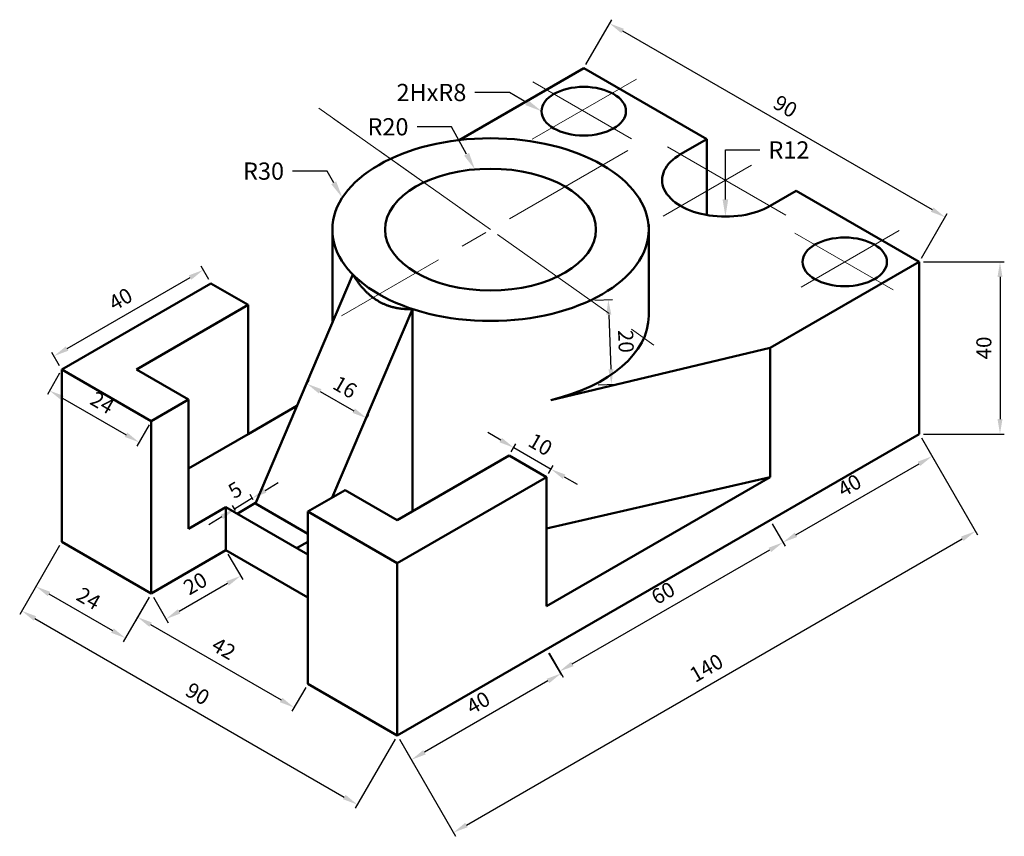
# Model space of a CAD drawing. Units: millimetres. Extents: x 2528 to 2757, y 816 to 1006.
import ezdxf
from ezdxf import colors
from ezdxf.entities.mleader import LeaderData, LeaderLine
from ezdxf.math import Vec2, Vec3

# ---------------------------------------------------------------- set-up
doc = ezdxf.new("R2010")
doc.units = ezdxf.units.MM
doc.linetypes.add('CENTER', pattern=[50.8, 31.75, -6.35, 6.35, -6.35])
for name, color, linetype, lineweight in [('M-CNTR', 4, 'CENTER', 18), ('M-DIMS', 3, 'Continuous', 25), ('M-OUTL', 7, 'Continuous', 50)]:
    doc.layers.add(name, color=color, linetype=linetype, lineweight=lineweight)
doc.styles.get("Standard").update_dxf_attribs({"font": 'arial.ttf'})
doc.dimstyles.new('AM_ISO$0', dxfattribs={"dimtxt": 3.5, "dimasz": 3.5, "dimexe": 1, "dimexo": 1, "dimgap": 1.5, "dimtad": 1, "dimdsep": 46, "dimtxsty": 'Standard', "dimcen": 0, "dimclrd": 256, "dimclre": 256, "dimclrt": 2, "dimadec": 0, "dimazin": 2, "dimtp": 0.1, "dimtm": 0.1, "dimtfac": 0.71, "dimtdec": 3, "dimtmove": 0, "dimatfit": 3, "dimfxl": 1, "dimlwd": -1, "dimlwe": -1, "dimarcsym": 1})

# ---------------------------------------------------------------- blocks, each defined once
blk = doc.blocks.new('*D3')
at = {"layer": 'Defpoints', "color": 0, "transparency": 16777216}
for p in [(2737.05, 909.84), (2750.08, 887.27), (2615.8, 839.84)]:
    blk.add_point(p, dxfattribs=at)
at = {"layer": 'M-DIMS', "color": 0, "linetype": 'ByBlock', "transparency": 16777216}
for p, q in [((2737.55, 908.97), (2750.58, 886.41)), ((2631.86, 819.02), (2747.04, 885.52)), ((2616.3, 838.97), (2629.33, 816.41))]:
    blk.add_line(p, q, dxfattribs=at)
at = {"layer": 'M-DIMS', "color": 0, "transparency": 16777216}
for points in [[(2746.75, 886.03), (2747.34, 885.02), (2750.08, 887.27)], [(2631.57, 819.53), (2632.15, 818.52), (2628.83, 817.27)]]:
    blk.add_solid(points, dxfattribs=at)
at = {"layer": 'M-DIMS', "color": 0, "transparency": 16777216, "insert": (2687.81, 855.12), "char_height": 3.5, "attachment_point": 5, "rotation": 30}
blk.add_mtext('140', dxfattribs=at)
blk = doc.blocks.new('*D4')
at = {"layer": 'Defpoints', "color": 0, "transparency": 16777216}
for p in [(2737.05, 949.84), (2737.05, 909.84), (2755.8, 909.84)]:
    blk.add_point(p, dxfattribs=at)
at = {"layer": 'M-DIMS', "color": 0, "linetype": 'ByBlock', "transparency": 16777216}
for p, q in [((2738.05, 949.84), (2756.8, 949.84)), ((2755.8, 946.34), (2755.8, 913.34)), ((2738.05, 909.84), (2756.8, 909.84))]:
    blk.add_line(p, q, dxfattribs=at)
at = {"layer": 'M-DIMS', "color": 0, "transparency": 16777216}
for points in [[(2755.22, 946.34), (2756.38, 946.34), (2755.8, 949.84)], [(2755.22, 913.34), (2756.38, 913.34), (2755.8, 909.84)]]:
    blk.add_solid(points, dxfattribs=at)
at = {"layer": 'M-DIMS', "color": 0, "transparency": 16777216, "insert": (2752.51, 929.84), "char_height": 3.5, "attachment_point": 5, "rotation": 90}
blk.add_mtext('40', dxfattribs=at)
blk = doc.blocks.new('*D5')
at = {"layer": 'Defpoints', "color": 0, "transparency": 16777216}
for p in [(2537.86, 884.84), (2558.64, 872.84), (2552.64, 862.45)]:
    blk.add_point(p, dxfattribs=at)
at = {"layer": 'M-DIMS', "color": 0, "linetype": 'ByBlock', "transparency": 16777216}
for p, q in [((2537.36, 883.97), (2531.36, 873.58)), ((2534.89, 872.7), (2549.61, 864.2)), ((2558.14, 871.97), (2552.14, 861.58))]:
    blk.add_line(p, q, dxfattribs=at)
at = {"layer": 'M-DIMS', "color": 0, "transparency": 16777216}
for points in [[(2535.18, 873.2), (2534.6, 872.19), (2531.86, 874.45)], [(2549.91, 864.7), (2549.32, 863.69), (2552.64, 862.45)]]:
    blk.add_solid(points, dxfattribs=at)
at = {"layer": 'M-DIMS', "color": 0, "transparency": 16777216, "insert": (2543.88, 871.27), "char_height": 3.5, "attachment_point": 5, "rotation": 330}
blk.add_mtext('24', dxfattribs=at)
blk = doc.blocks.new('*D6')
at = {"layer": 'Defpoints', "color": 0, "transparency": 16777216}
for p in [(2575.97, 882.84), (2558.64, 872.84), (2562.08, 866.89)]:
    blk.add_point(p, dxfattribs=at)
at = {"layer": 'M-DIMS', "color": 0, "linetype": 'ByBlock', "transparency": 16777216}
for p, q in [((2576.47, 881.97), (2579.9, 876.03)), ((2576.37, 875.14), (2565.11, 868.64)), ((2559.14, 871.97), (2562.58, 866.03))]:
    blk.add_line(p, q, dxfattribs=at)
at = {"layer": 'M-DIMS', "color": 0, "transparency": 16777216}
for points in [[(2576.08, 875.65), (2576.66, 874.64), (2579.4, 876.89)], [(2564.82, 869.15), (2565.4, 868.14), (2562.08, 866.89)]]:
    blk.add_solid(points, dxfattribs=at)
at = {"layer": 'M-DIMS', "color": 0, "transparency": 16777216, "insert": (2569.1, 874.74), "char_height": 3.5, "attachment_point": 5, "rotation": 30}
blk.add_mtext('20', dxfattribs=at)
blk = doc.blocks.new('*D7')
at = {"layer": 'Defpoints', "color": 0, "transparency": 16777216}
for p in [(2659.1, 994.84), (2743.05, 960.23), (2737.05, 949.84)]:
    blk.add_point(p, dxfattribs=at)
at = {"layer": 'M-DIMS', "color": 0, "linetype": 'ByBlock', "transparency": 16777216}
for p, q in [((2659.6, 995.71), (2665.6, 1006.1)), ((2668.13, 1003.48), (2740.01, 961.98)), ((2737.55, 950.71), (2743.55, 961.1))]:
    blk.add_line(p, q, dxfattribs=at)
at = {"layer": 'M-DIMS', "color": 0, "transparency": 16777216}
for points in [[(2668.43, 1003.99), (2667.84, 1002.98), (2665.1, 1005.23)], [(2740.31, 962.49), (2739.72, 961.48), (2743.05, 960.23)]]:
    blk.add_solid(points, dxfattribs=at)
at = {"layer": 'M-DIMS', "color": 0, "transparency": 16777216, "insert": (2705.72, 985.58), "char_height": 3.5, "attachment_point": 5, "rotation": 330}
blk.add_mtext('90', dxfattribs=at)
blk = doc.blocks.new('*D8')
at = {"layer": 'Defpoints', "color": 0, "transparency": 16777216}
for p in [(2578.01, 892.42), (2582.83, 893.74), (2578.74, 891.24)]:
    blk.add_point(p, dxfattribs=at)
at = {"layer": 'M-DIMS', "color": 0, "linetype": 'ByBlock', "transparency": 16777216}
for p, q in [((2585.1, 896.74), (2588.09, 898.56)), ((2582.11, 894.92), (2578.01, 892.42)), ((2582.31, 894.59), (2581.59, 895.77)), ((2578.22, 892.09), (2577.49, 893.28)), ((2575.03, 890.6), (2572.04, 888.78))]:
    blk.add_line(p, q, dxfattribs=at)
at = {"layer": 'M-DIMS', "color": 0, "transparency": 16777216}
for points in [[(2584.8, 897.24), (2585.4, 896.24), (2582.11, 894.92)], [(2574.72, 891.1), (2575.33, 890.1), (2578.01, 892.42)]]:
    blk.add_solid(points, dxfattribs=at)
at = {"layer": 'M-DIMS', "color": 0, "transparency": 16777216, "insert": (2578.36, 896.47), "char_height": 3.5, "attachment_point": 5, "rotation": 31.3574}
blk.add_mtext('5', dxfattribs=at)
blk = doc.blocks.new('*D9')
at = {"layer": 'Defpoints', "color": 0, "transparency": 16777216}
for p in [(2594.16, 920.31), (2608.71, 913.51), (2608.02, 912.31)]:
    blk.add_point(p, dxfattribs=at)
at = {"layer": 'M-DIMS', "color": 0, "linetype": 'ByBlock', "transparency": 16777216}
for p, q in [((2594.66, 921.18), (2595.35, 922.38)), ((2597.89, 919.76), (2605.68, 915.26)), ((2608.52, 913.18), (2609.21, 914.38))]:
    blk.add_line(p, q, dxfattribs=at)
at = {"layer": 'M-DIMS', "color": 0, "transparency": 16777216}
for points in [[(2598.18, 920.27), (2597.59, 919.26), (2594.85, 921.51)], [(2605.97, 915.77), (2605.39, 914.76), (2608.71, 913.51)]]:
    blk.add_solid(points, dxfattribs=at)
at = {"layer": 'M-DIMS', "color": 0, "transparency": 16777216, "insert": (2603.43, 920.36), "char_height": 3.5, "attachment_point": 5, "rotation": 330}
blk.add_mtext('16', dxfattribs=at)
blk = doc.blocks.new('*D10')
at = {"layer": 'Defpoints', "color": 0, "transparency": 16777216}
for p in [(2570.7, 947.96), (2572.5, 944.84), (2537.86, 924.84)]:
    blk.add_point(p, dxfattribs=at)
at = {"layer": 'M-DIMS', "color": 0, "linetype": 'ByBlock', "transparency": 16777216}
for p, q in [((2572, 945.71), (2570.2, 948.82)), ((2539.09, 929.71), (2567.67, 946.21)), ((2537.36, 925.71), (2535.56, 928.82))]:
    blk.add_line(p, q, dxfattribs=at)
at = {"layer": 'M-DIMS', "color": 0, "transparency": 16777216}
for points in [[(2567.38, 946.71), (2567.96, 945.7), (2570.7, 947.96)], [(2538.8, 930.21), (2539.38, 929.2), (2536.06, 927.96)]]:
    blk.add_solid(points, dxfattribs=at)
at = {"layer": 'M-DIMS', "color": 0, "transparency": 16777216, "insert": (2551.74, 940.8), "char_height": 3.5, "attachment_point": 5, "rotation": 30}
blk.add_mtext('40', dxfattribs=at)
blk = doc.blocks.new('*D11')
at = {"layer": 'Defpoints', "color": 0, "transparency": 16777216}
for p in [(2537.86, 924.84), (2558.64, 912.84), (2555.81, 907.93)]:
    blk.add_point(p, dxfattribs=at)
at = {"layer": 'M-DIMS', "color": 0, "linetype": 'ByBlock', "transparency": 16777216}
for p, q in [((2537.36, 923.97), (2534.53, 919.06)), ((2538.06, 918.18), (2552.78, 909.68)), ((2558.14, 911.97), (2555.31, 907.06))]:
    blk.add_line(p, q, dxfattribs=at)
at = {"layer": 'M-DIMS', "color": 0, "transparency": 16777216}
for points in [[(2538.35, 918.69), (2537.77, 917.68), (2535.03, 919.93)], [(2553.07, 910.19), (2552.49, 909.18), (2555.81, 907.93)]]:
    blk.add_solid(points, dxfattribs=at)
at = {"layer": 'M-DIMS', "color": 0, "transparency": 16777216, "insert": (2547.05, 916.75), "char_height": 3.5, "attachment_point": 5, "rotation": 330}
blk.add_mtext('24', dxfattribs=at)
blk = doc.blocks.new('*D12')
at = {"layer": 'Defpoints', "color": 0, "transparency": 16777216}
for p in [(2660.68, 940.9), (2661.43, 921.26), (2665.55, 921.42)]:
    blk.add_point(p, dxfattribs=at)
at = {"layer": 'M-DIMS', "color": 0, "linetype": 'ByBlock', "transparency": 16777216}
for p, q in [((2661.68, 940.94), (2665.81, 941.1)), ((2664.94, 937.56), (2665.42, 924.92)), ((2662.43, 921.3), (2666.55, 921.46))]:
    blk.add_line(p, q, dxfattribs=at)
at = {"layer": 'M-DIMS', "color": 0, "transparency": 16777216}
for points in [[(2665.52, 937.58), (2664.36, 937.54), (2664.81, 941.06)], [(2666, 924.94), (2664.84, 924.9), (2665.55, 921.42)]]:
    blk.add_solid(points, dxfattribs=at)
at = {"layer": 'M-DIMS', "color": 0, "transparency": 16777216, "insert": (2668.46, 931.36), "char_height": 3.5, "attachment_point": 5, "rotation": 272.1711}
blk.add_mtext('20', dxfattribs=at)
blk = doc.blocks.new('*D13')
at = {"layer": 'Defpoints', "color": 0, "transparency": 16777216}
for p in [(2737.05, 909.84), (2740.02, 904.69), (2702.4, 889.84)]:
    blk.add_point(p, dxfattribs=at)
at = {"layer": 'M-DIMS', "color": 0, "linetype": 'ByBlock', "transparency": 16777216}
for p, q in [((2737.55, 908.97), (2740.52, 903.82)), ((2708.41, 886.44), (2736.99, 902.94)), ((2702.9, 888.97), (2705.88, 883.82))]:
    blk.add_line(p, q, dxfattribs=at)
at = {"layer": 'M-DIMS', "color": 0, "transparency": 16777216}
for points in [[(2736.7, 903.44), (2737.28, 902.43), (2740.02, 904.69)], [(2708.12, 886.94), (2708.7, 885.93), (2705.38, 884.69)]]:
    blk.add_solid(points, dxfattribs=at)
at = {"layer": 'M-DIMS', "color": 0, "transparency": 16777216, "insert": (2721.06, 897.53), "char_height": 3.5, "attachment_point": 5, "rotation": 30}
blk.add_mtext('40', dxfattribs=at)
blk = doc.blocks.new('*D14')
at = {"layer": 'Defpoints', "color": 0, "transparency": 16777216}
for p in [(2702.4, 889.84), (2705.38, 884.69), (2650.44, 859.84)]:
    blk.add_point(p, dxfattribs=at)
at = {"layer": 'M-DIMS', "color": 0, "linetype": 'ByBlock', "transparency": 16777216}
for p, q in [((2702.9, 888.97), (2705.88, 883.82)), ((2656.45, 856.44), (2702.35, 882.94)), ((2650.94, 858.97), (2653.92, 853.82))]:
    blk.add_line(p, q, dxfattribs=at)
at = {"layer": 'M-DIMS', "color": 0, "transparency": 16777216}
for points in [[(2702.06, 883.44), (2702.64, 882.43), (2705.38, 884.69)], [(2656.16, 856.94), (2656.74, 855.93), (2653.42, 854.69)]]:
    blk.add_solid(points, dxfattribs=at)
at = {"layer": 'M-DIMS', "color": 0, "transparency": 16777216, "insert": (2677.76, 872.53), "char_height": 3.5, "attachment_point": 5, "rotation": 30}
blk.add_mtext('60', dxfattribs=at)
blk = doc.blocks.new('*D15')
at = {"layer": 'Defpoints', "color": 0, "transparency": 16777216}
for p in [(2641.78, 904.84), (2651.51, 901.69), (2650.44, 899.84)]:
    blk.add_point(p, dxfattribs=at)
at = {"layer": 'M-DIMS', "color": 0, "linetype": 'ByBlock', "transparency": 16777216}
for p, q in [((2639.82, 908.44), (2636.79, 910.19)), ((2642.28, 905.71), (2643.35, 907.55)), ((2642.85, 906.69), (2651.51, 901.69)), ((2650.94, 900.71), (2652.01, 902.55)), ((2654.54, 899.94), (2657.57, 898.19))]:
    blk.add_line(p, q, dxfattribs=at)
at = {"layer": 'M-DIMS', "color": 0, "transparency": 16777216}
for points in [[(2640.11, 908.94), (2639.53, 907.93), (2642.85, 906.69)], [(2654.83, 900.44), (2654.25, 899.43), (2651.51, 901.69)]]:
    blk.add_solid(points, dxfattribs=at)
at = {"layer": 'M-DIMS', "color": 0, "transparency": 16777216, "insert": (2648.82, 907.04), "char_height": 3.5, "attachment_point": 5, "rotation": 330}
blk.add_mtext('10', dxfattribs=at)
blk = doc.blocks.new('*D16')
at = {"layer": 'Defpoints', "color": 0, "transparency": 16777216}
for p in [(2537.86, 884.84), (2615.8, 839.84), (2606.53, 823.77)]:
    blk.add_point(p, dxfattribs=at)
at = {"layer": 'M-DIMS', "color": 0, "linetype": 'ByBlock', "transparency": 16777216}
for p, q in [((2537.36, 883.97), (2528.08, 867.91)), ((2531.61, 867.02), (2603.49, 825.52)), ((2615.3, 838.97), (2606.03, 822.91))]:
    blk.add_line(p, q, dxfattribs=at)
at = {"layer": 'M-DIMS', "color": 0, "transparency": 16777216}
for points in [[(2531.91, 867.53), (2531.32, 866.52), (2528.58, 868.77)], [(2603.79, 826.03), (2603.2, 825.02), (2606.53, 823.77)]]:
    blk.add_solid(points, dxfattribs=at)
at = {"layer": 'M-DIMS', "color": 0, "transparency": 16777216, "insert": (2569.2, 849.12), "char_height": 3.5, "attachment_point": 5, "rotation": 330}
blk.add_mtext('90', dxfattribs=at)
blk = doc.blocks.new('*D17')
at = {"layer": 'Defpoints', "color": 0, "transparency": 16777216}
for p in [(2558.64, 872.84), (2595.02, 851.84), (2591.83, 846.32)]:
    blk.add_point(p, dxfattribs=at)
at = {"layer": 'M-DIMS', "color": 0, "linetype": 'ByBlock', "transparency": 16777216}
for p, q in [((2558.14, 871.97), (2554.96, 866.45)), ((2558.49, 865.57), (2588.8, 848.07)), ((2594.52, 850.97), (2591.33, 845.45))]:
    blk.add_line(p, q, dxfattribs=at)
at = {"layer": 'M-DIMS', "color": 0, "transparency": 16777216}
for points in [[(2558.78, 866.08), (2558.2, 865.06), (2555.46, 867.32)], [(2589.09, 848.58), (2588.51, 847.56), (2591.83, 846.32)]]:
    blk.add_solid(points, dxfattribs=at)
at = {"layer": 'M-DIMS', "color": 0, "transparency": 16777216, "insert": (2575.27, 859.64), "char_height": 3.5, "attachment_point": 5, "rotation": 330}
blk.add_mtext('42', dxfattribs=at)
blk = doc.blocks.new('*D18')
at = {"layer": 'Defpoints', "color": 0, "transparency": 16777216}
for p in [(2650.56, 859.9), (2615.8, 839.84), (2619.07, 834.17)]:
    blk.add_point(p, dxfattribs=at)
at = {"layer": 'M-DIMS', "color": 0, "linetype": 'ByBlock', "transparency": 16777216}
for p, q in [((2651.06, 859.04), (2654.33, 853.37)), ((2650.79, 852.49), (2622.1, 835.92)), ((2616.3, 838.97), (2619.57, 833.31))]:
    blk.add_line(p, q, dxfattribs=at)
at = {"layer": 'M-DIMS', "color": 0, "transparency": 16777216}
for points in [[(2650.5, 852.99), (2651.09, 851.98), (2653.83, 854.24)], [(2621.81, 836.43), (2622.4, 835.42), (2619.07, 834.17)]]:
    blk.add_solid(points, dxfattribs=at)
at = {"layer": 'M-DIMS', "color": 0, "transparency": 16777216, "insert": (2634.81, 847.05), "char_height": 3.5, "attachment_point": 5, "rotation": 30}
blk.add_mtext('40', dxfattribs=at)

msp = doc.modelspace()

# ---------------------------------------------------------------- linework, layer by layer
at = {"layer": 'M-CNTR'}
for p, q in [((2647.134, 978.352), (2671.327, 992.32)), ((2670.168, 978.452), (2647.307, 991.651)), ((2637.453, 957.34), (2597.606, 985.534)), ((2597.606, 985.534), (2678.628, 928.206)), ((2669.338, 975.748), (2602.812, 937.34)), ((2678.589, 976.59), (2708.652, 959.233)), ((2698.075, 972.34), (2677.527, 960.476)), ((2674.195, 958.553), (2674.138, 958.52)), ((2708.114, 956.547), (2730.951, 943.362)), ((2732.384, 957.15), (2709.608, 944))]:
    msp.add_line(p, q, dxfattribs=at)
at = {"layer": 'M-OUTL'}
for p, q in [((2659.104, 994.84), (2630.164, 978.131)), ((2687.682, 978.34), (2659.104, 994.84)), ((2681.62, 974.84), (2687.682, 978.34)), ((2687.682, 960.731), (2687.682, 978.34)), ((2702.405, 962.84), (2708.467, 966.34)), ((2737.046, 949.84), (2708.467, 966.34)), ((2674.195, 937.34), (2674.195, 958.553)), ((2600.711, 937.34), (2600.711, 957.34)), ((2737.046, 949.84), (2702.405, 929.84)), ((2737.046, 909.84), (2737.046, 949.84)), ((2537.86, 924.84), (2572.501, 944.84)), ((2572.501, 944.84), (2581.161, 939.84)), ((2582.833, 893.737), (2605.485, 946.883)), ((2581.161, 939.84), (2555.181, 924.84)), ((2581.161, 939.84), (2581.161, 909.84)), ((2619.341, 938.883), (2600.685, 895.112)), ((2619.341, 938.883), (2619.341, 891.883)), ((2702.405, 929.84), (2651.443, 917.724)), ((2702.405, 929.84), (2702.405, 899.84)), ((2558.645, 912.84), (2537.86, 924.84)), ((2537.86, 924.84), (2537.86, 884.84)), ((2555.181, 924.84), (2567.305, 917.84)), ((2567.305, 917.84), (2558.645, 912.84)), ((2567.305, 917.84), (2567.305, 887.84)), ((2581.161, 909.84), (2592.482, 916.376)), ((2558.645, 872.84), (2558.645, 912.84)), ((2581.161, 909.84), (2567.305, 901.84)), ((2615.802, 839.84), (2737.046, 909.84)), ((2641.783, 904.84), (2615.802, 889.84)), ((2650.443, 899.84), (2641.783, 904.84)), ((2615.802, 879.84), (2650.443, 899.84)), ((2702.405, 899.84), (2650.443, 869.84)), ((2650.443, 869.84), (2650.443, 899.84)), ((2702.405, 899.84), (2650.443, 887.925)), ((2603.678, 896.84), (2595.018, 891.84)), ((2615.802, 889.84), (2603.678, 896.84)), ((2567.305, 887.84), (2575.965, 892.84)), ((2575.965, 892.84), (2575.965, 882.84)), ((2575.965, 892.84), (2595.018, 881.84)), ((2578.563, 891.339), (2582.893, 893.839)), ((2595.018, 886.702), (2582.833, 893.737)), ((2589.702, 889.771), (2589.822, 889.84)), ((2595.018, 891.84), (2615.802, 879.84)), ((2595.018, 851.84), (2595.018, 891.84)), ((2537.86, 884.84), (2558.645, 872.84)), ((2592.42, 883.339), (2595.018, 884.839)), ((2575.965, 882.84), (2558.645, 872.84)), ((2595.018, 871.84), (2575.965, 882.84)), ((2615.802, 879.84), (2615.802, 839.84)), ((2615.802, 839.84), (2595.018, 851.84))]:
    msp.add_line(p, q, dxfattribs=at)
msp.add_lwpolyline([(2619.341, 938.883), (2619.163, 938.879), (2618.986, 938.876), (2618.808, 938.873), (2618.63, 938.869), (2618.452, 938.866), (2618.275, 938.862), (2618.097, 938.861), (2617.924, 938.871), (2617.75, 938.882), (2617.577, 938.892), (2617.403, 938.902), (2617.23, 938.912), (2617.056, 938.923), (2616.884, 938.937), (2616.715, 938.961), (2616.545, 938.984), (2616.376, 939.008), (2616.207, 939.032), (2616.038, 939.056), (2615.869, 939.08), (2615.702, 939.109), (2615.537, 939.147), (2615.373, 939.184), (2615.209, 939.222), (2615.044, 939.259), (2614.88, 939.297), (2614.715, 939.334), (2614.554, 939.379), (2614.394, 939.43), (2614.235, 939.481), (2614.075, 939.532), (2613.916, 939.583), (2613.756, 939.634), (2613.597, 939.685), (2613.441, 939.745), (2613.287, 939.81), (2613.132, 939.874), (2612.978, 939.938), (2612.824, 940.003), (2612.67, 940.067), (2612.515, 940.132), (2612.366, 940.207), (2612.217, 940.285), (2612.068, 940.363), (2611.919, 940.441), (2611.77, 940.518), (2611.621, 940.596), (2611.472, 940.674), (2611.329, 940.765), (2611.186, 940.856), (2611.042, 940.947), (2610.899, 941.038), (2610.756, 941.128), (2610.613, 941.219), (2610.47, 941.312), (2610.333, 941.416), (2610.195, 941.52), (2610.058, 941.624), (2609.921, 941.728), (2609.783, 941.832), (2609.646, 941.936), (2609.51, 942.044), (2609.379, 942.161), (2609.247, 942.278), (2609.116, 942.395), (2608.985, 942.512), (2608.853, 942.629), (2608.722, 942.746), (2608.593, 942.869), (2608.468, 942.998), (2608.343, 943.128), (2608.218, 943.258), (2608.093, 943.387), (2607.968, 943.517), (2607.843, 943.647), (2607.721, 943.784), (2607.603, 943.926), (2607.484, 944.068), (2607.365, 944.211), (2607.247, 944.353), (2607.128, 944.495), (2607.009, 944.638), (2606.895, 944.789), (2606.783, 944.944), (2606.671, 945.098), (2606.559, 945.253), (2606.447, 945.408), (2606.335, 945.562), (2606.223, 945.717), (2606.117, 945.882), (2606.011, 946.049), (2605.906, 946.215), (2605.801, 946.382), (2605.695, 946.549), (2605.59, 946.716), (2605.485, 946.883)], dxfattribs=at)
for centre, major_axis in [((2659.104, 984.84), (-9.798, 0)), ((2637.453, 957.34), (-36.742, 0)), ((2637.453, 957.34), (-24.495, 0)), ((2719.727, 949.842), (-9.798, 0))]:
    msp.add_ellipse(centre, major_axis=major_axis, ratio=0.5773503, dxfattribs=at)
for centre, major_axis, start_param, end_param in [((2692.013, 968.84), (-14.697, 0), 5.4977871, 8.6393798), ((2637.453, 937.34), (-36.742, 0), 6.2831853, 6.35183), ((2637.453, 937.339), (-36.742, 0), 1.9614034, 3.1415927)]:
    msp.add_ellipse(centre, major_axis=major_axis, ratio=0.5773503, start_param=start_param, end_param=end_param, dxfattribs=at)

# ---------------------------------------------------------------- dimensions: what is measured, and where the dimension line sits
at = {"layer": 'M-DIMS'}
for p1, p2, distance, override, picture, middle in [((2659.104, 994.84), (2737.046, 949.84), 12, {"dimclrd": 0, "dimclre": 0, "dimclrt": 0}, '*D7', (2705.718, 985.578)), ((2737.046, 949.84), (2737.046, 909.84), 18.754, {"dimclrd": 0, "dimclre": 0, "dimclrt": 0}, '*D4', (2752.513, 929.84)), ((2537.86, 924.84), (2572.501, 944.84), 3.6, {"dimclrd": 0, "dimclre": 0, "dimclrt": 0}, '*D10', (2551.737, 940.804)), ((2537.86, 924.84), (2558.645, 912.84), -5.668, {"dimclrd": 0, "dimclre": 0, "dimclrt": 0}, '*D11', (2547.047, 916.751)), ((2594.159, 920.31), (2608.015, 912.31), 1.391, {"dimpost": '', "dimclrd": 0, "dimclre": 0, "dimclrt": 0}, '*D9', (2603.426, 920.36)), ((2641.783, 904.84), (2650.443, 899.84), 2.135, {"dimpost": '', "dimclrd": 0, "dimclre": 0, "dimclrt": 0}, '*D15', (2648.824, 907.035)), ((2615.802, 839.84), (2737.046, 909.84), -26.059, {"dimpost": '', "dimclrd": 0, "dimclre": 0, "dimclrt": 0}, '*D3', (2687.81, 855.118)), ((2702.405, 889.84), (2737.046, 909.84), -5.95, {"dimpost": '', "dimclrd": 0, "dimclre": 0, "dimclrt": 0}, '*D13', (2721.057, 897.534)), ((2650.443, 859.84), (2702.405, 889.84), -5.95, {"dimclrd": 0, "dimclre": 0, "dimclrt": 0}, '*D14', (2677.756, 872.534)), ((2537.86, 884.84), (2615.802, 839.84), -18.554, {"dimclrd": 0, "dimclre": 0, "dimclrt": 0}, '*D16', (2569.198, 849.118)), ((2537.86, 884.84), (2558.645, 872.84), -12, {"dimclrd": 0, "dimclre": 0, "dimclrt": 0}, '*D5', (2543.881, 871.268)), ((2575.965, 882.84), (2558.645, 872.84), 6.869, {"dimclrd": 0, "dimclre": 0, "dimclrt": 0}, '*D6', (2569.096, 874.738)), ((2558.645, 872.84), (2595.018, 851.84), -6.373, {"dimclrd": 0, "dimclre": 0, "dimclrt": 0}, '*D17', (2575.273, 859.641))]:
    dim = msp.add_aligned_dim(p1=p1, p2=p2, distance=distance, dimstyle='AM_ISO$0', override=override, dxfattribs=at)
    dim.commit()
    dim.dimension.update_dxf_attribs({"geometry": picture, "text_midpoint": middle})
for p1, p2, distance, text, picture, middle in [((2660.682, 940.904), (2661.426, 921.264), 4.129, '20', '*D12', (2668.465, 931.365)), ((2650.555, 859.904), (2615.802, 839.84), 6.541, '40', '*D18', (2634.806, 847.054))]:
    dim = msp.add_aligned_dim(p1=p1, p2=p2, distance=distance, text=text, dimstyle='AM_ISO$0', override={"dimpost": '', "dimclrd": 0, "dimclre": 0, "dimclrt": 0}, dxfattribs=at)
    dim.commit()
    dim.dimension.update_dxf_attribs({"geometry": picture, "text_midpoint": middle})
dim = msp.add_linear_dim(base=(2578.014, 892.424), p1=(2582.833, 893.737), p2=(2578.736, 891.24), angle=211.35738, text='5', dimstyle='AM_ISO$0', override={"dimclrd": 0, "dimclre": 0, "dimclrt": 0}, dxfattribs=at)
dim.commit()
dim.dimension.update_dxf_attribs({"geometry": '*D8', "text_midpoint": (2580.063, 893.672), "dimtype": 161})

# ---------------------------------------------------------------- leaders
ml = msp.add_multileader_mtext('Standard', dxfattribs=at)
ml.set_content('{\\C2;2HxR8}', color=256)
ml.set_leader_properties()
ml.build(insert=Vec2(0, 0))
ctx = ml.context
ctx.base_point, ctx.plane_origin = Vec3(2613.162, 989.154), Vec3(2649.306, 984.84)
ctx.text_align_type = 2
notes = []
notes.append((ctx, [(0, (1, 1, 0), (2641.833, 989.154), (-1, 0), 8, [(0, [(2649.306, 984.84)], 0, [])])]))
ctx.mtext.insert, ctx.mtext.alignment, ctx.mtext.flow_direction = Vec3(2631.833, 991.188), 3, 5
ml = msp.add_multileader_mtext('Standard', dxfattribs=at)
ml.set_content('{\\C2;R20}', color=256)
ml.set_leader_properties()
ml.build(insert=Vec2(0, 0))
ctx = ml.context
ctx.base_point, ctx.plane_origin = Vec3(2606.857, 981.185), Vec3(2633.827, 971.326)
ctx.text_align_type = 2
notes.append((ctx, [(0, (1, 1, 0), (2628.401, 981.185), (-1, 0), 8, [(0, [(2633.827, 971.326)], 0, [])])]))
ctx.mtext.insert, ctx.mtext.alignment, ctx.mtext.flow_direction = Vec3(2618.401, 983.219), 3, 5
ml = msp.add_multileader_mtext('Standard', dxfattribs=at)
ml.set_content('{\\C2;R12}', color=256)
ml.set_leader_properties()
ml.build(insert=Vec2(0, 0))
ctx = ml.context
ctx.base_point, ctx.plane_origin = Vec3(2700.013, 975.84), Vec3(2692.013, 960.354)
notes.append((ctx, [(0, (1, 1, 0), (2692.013, 975.84), (1, 0), 8, [(0, [(2692.013, 960.354)], 0, [])])]))
ctx.mtext.insert, ctx.mtext.flow_direction = Vec3(2702.013, 977.84), 5
ml = msp.add_multileader_mtext('Standard', dxfattribs=at)
ml.set_content('{\\C2;R30}', color=256)
ml.set_leader_properties()
ml.build(insert=Vec2(0, 0))
ctx = ml.context
ctx.base_point, ctx.plane_origin = Vec3(2577.942, 970.891), Vec3(2603.029, 964.755)
ctx.text_align_type = 2
notes.append((ctx, [(0, (1, 1, 0), (2599.486, 970.891), (-1, 0), 8, [(0, [(2603.029, 964.755)], 0, [])])]))
ctx.mtext.insert, ctx.mtext.alignment, ctx.mtext.flow_direction = Vec3(2589.486, 972.927), 3, 5
for ctx, leaders in notes:
    for number, flags, end, landing, length, lines in leaders:
        leader = LeaderData()
        leader.index, (leader.has_last_leader_line, leader.has_dogleg_vector, leader.attachment_direction) = number, flags
        leader.last_leader_point, leader.dogleg_vector, leader.dogleg_length = Vec3(end), Vec3(landing), length
        for number, points, colour, breaks in lines:
            line = LeaderLine()
            line.index, line.vertices, line.color, line.breaks = number, Vec3.list(points), colors.encode_raw_color(colour), breaks
            leader.lines.append(line)
        ctx.leaders.append(leader)

doc.saveas('drawing.dxf')
